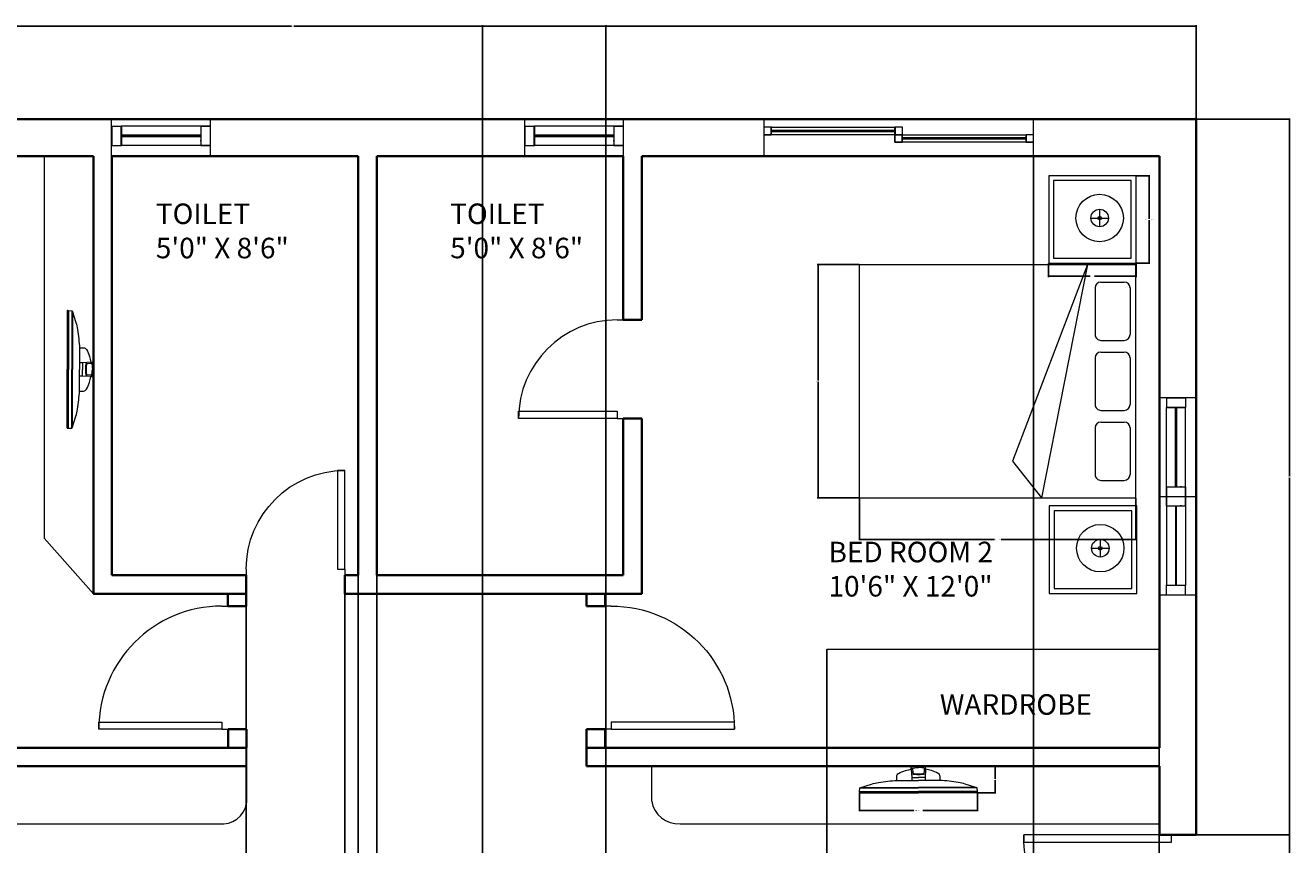
# Model space of a CAD drawing. Units: inches. Extents: x 1723 to 2209, y 1326 to 1810.
# Tile 6 of 6: x 1901 to 2209, y 1610 to 1810. Entities that reach past the tile are written whole.
import ezdxf

# ---------------------------------------------------------------- set-up
doc = ezdxf.new("R2010")
doc.units = ezdxf.units.IN
doc.layers.get('Defpoints').update_dxf_attribs({"color": 255})
for name, color, linetype, lineweight in [('A-ANNO-DIMS', 2, 'Continuous', 18), ('A-ANNO-TEXT', 7, 'Continuous', 18), ('A-AREA-IDEN', 7, 'Continuous', 18), ('A-DOOR', 3, 'Continuous', 18), ('A-EQPM', 8, 'Continuous', 13), ('A-FLOR-CASE', 9, 'Continuous', 18), ('A-FURN', 8, 'Continuous', 13), ('A-GLAZ', 4, 'Continuous', 18), ('A-WALL', 7, 'Continuous', 35), ('Sliding Door', 3, 'Continuous', 18)]:
    doc.layers.add(name, color=color, linetype=linetype, lineweight=lineweight)
doc.styles.get("Standard").update_dxf_attribs({"font": 'arial.ttf'})
doc.dimstyles.get("Standard").update_dxf_attribs({"dimtxt": 0.18, "dimasz": 0.18, "dimexe": 0.18, "dimexo": 0.0625, "dimgap": 0.09, "dimtad": 0, "dimtih": 1, "dimtoh": 1, "dimdec": 4, "dimzin": 0, "dimdsep": 46, "dimtxsty": 'Standard', "dimcen": 0.09, "dimadec": 0, "dimazin": 0, "dimtfac": 1, "dimtdec": 4, "dimtofl": 0, "dimtmove": 0, "dimatfit": 3, "dimfxl": 1, "dimtolj": 1, "dimtzin": 0, "dimarcsym": 0})

# ---------------------------------------------------------------- blocks, each defined once
blk = doc.blocks.new('B1')
at = {"color": 0}
for points in [[(-24.5, 37.9), (-24.5, 43.2, -0.236854), (-23.9, 44.5, -0.069077), (0, 47.8, -0.069077)], [(-24.5, 37.7), (-24.5, 38.9, -0.236854), (-23.9, 40.2, -0.069077), (0, 43.6, -0.069077)], [(24.5, 37.9), (24.5, 43.2, 0.236854), (23.9, 44.5, 0.069077), (0, 47.8, 0.069077)], [(24.5, 37.7), (24.5, 38.9, 0.236854), (23.9, 40.2, 0.069077), (0, 43.6, 0.069077)], [(-200, -38.4), (-200, -37.7), (-199.2, -25.8, -0.303983), (-198.5, -24.8), (-159.1, -12.4, -0.039649), (-135.4, -7, -0.017831), (-72.5, 0), (0, 0)], [(-73.6, -0.1), (-73.6, 13.1, -0.272026), (-67.3, 23.9, -0.059641), (-43.9, 33.5, -0.024069), (-24.5, 37.9), (-22.7, 10), (-22.7, 0)], [(200, -38.4), (200, -37.7), (199.2, -25.8, 0.303983), (198.5, -24.8), (159.1, -12.4, 0.039649), (135.4, -7, 0.017831), (72.5, 0), (0, 0)], [(73.6, -0.1), (73.6, 13.1, 0.272026), (67.3, 23.9, 0.059641), (43.9, 33.5, 0.024069), (24.5, 37.9), (22.7, 10), (22.7, 0)]]:
    blk.add_lwpolyline(points, format="xyb", dxfattribs=at)
for points in [[(-22.7, 10), (0, 10)], [(-19.8, 40.1), (-18.9, 26.4)], [(22.7, 10), (0, 10)], [(19.8, 40.1), (18.9, 26.4)], [(-200, -37.8), (0, -37.8)], [(-200, -41.4), (-200, -38.4), (200, -38.4)], [(-200, -38.4), (0, -38.4)], [(200, -41.4), (200, -38.4), (-200, -38.4)], [(-199.2, -25.8), (0, -25.8)], [(-198.9, -42.4), (0, -42.4)], [(-196.3, -24.2), (0, -24.2)], [(196.3, -24.2), (0, -24.2)], [(199.2, -25.8), (0, -25.8)], [(200, -37.8), (0, -37.8)], [(200, -38.4), (0, -38.4)], [(198.9, -42.4), (0, -42.4)]]:
    blk.add_lwpolyline(points, dxfattribs=at)
for centre, radius, start, end in [((0, 150), 130, 259.5789, 270), ((-15.4, 26.6), 3.53, 183.678, 262.9963), ((0, 152.2), 130, 262.9963, 270), ((0, 152.2), 130, 270, 277.0037), ((0, 150), 130, 270, 280.4211), ((15.4, 26.6), 3.53, 277.0037, 356.322), ((-198.9, -41.4), 1.06, 180, 270), ((198.9, -41.4), 1.06, 270, 0)]:
    blk.add_arc(centre, radius, start, end, dxfattribs=at)
blk = doc.blocks.new('A$C793B20D3')
for p, q in [((0.625, -0.395), (0.625, 1.975)), ((2.625, 1.975), (0.625, 1.975)), ((2.625, -0.395), (2.625, 1.975)), ((0.775, 1.675), (0.775, 1.875)), ((0.825, 1.925), (1.225, 1.925)), ((1.275, 1.675), (1.275, 1.875)), ((1.375, 1.675), (1.375, 1.875)), ((1.425, 1.925), (1.825, 1.925)), ((1.875, 1.675), (1.875, 1.875)), ((1.975, 1.675), (1.975, 1.875)), ((2.025, 1.925), (2.425, 1.925)), ((2.475, 1.675), (2.475, 1.875)), ((0.626, 1.56), (2.311, 0.917)), ((0.626, 1.56), (2.625, 1.165)), ((0.825, 1.625), (1.225, 1.625)), ((1.425, 1.625), (1.825, 1.625)), ((2.025, 1.625), (2.425, 1.625)), ((2.311, 0.917), (2.625, 1.165)), ((2.625, -0.395), (0.625, -0.395))]:
    blk.add_line(p, q)
for centre, start, end in [((0.825, 1.875), 90, 180), ((1.225, 1.875), 0, 90), ((1.425, 1.875), 90, 180), ((1.825, 1.875), 0, 90), ((2.025, 1.875), 90, 180), ((2.425, 1.875), 0, 90), ((0.825, 1.675), 180, 270), ((1.225, 1.675), 270, 0), ((1.425, 1.675), 180, 270), ((1.825, 1.675), 270, 0), ((2.025, 1.675), 180, 270), ((2.425, 1.675), 270, 0)]:
    blk.add_arc(centre, 0.05, start, end)
blk = doc.blocks.new('*U40')
for p, q in [((0, 0), (0, -6)), ((30, 0), (30, -6))]:
    blk.add_line(p, q)
blk.add_lwpolyline([(0, 0), (0, 30), (1.75, 30), (1.75, 0)], close=True)
blk.add_arc((0, 0), 30, 0, 90)
blk = doc.blocks.new('*U39')
for p, q in [((0, 0), (0, -6)), ((24, 0), (24, -6))]:
    blk.add_line(p, q)
blk.add_lwpolyline([(0, 0), (0, 24), (1.75, 24), (1.75, 0)], close=True)
blk.add_arc((0, 0), 24, 0, 90)
blk = doc.blocks.new('*U41')
for p, q in [((0, 0), (0, -6)), ((36, 0), (36, -6))]:
    blk.add_line(p, q)
blk.add_lwpolyline([(0, 0), (0, 36), (1.75, 36), (1.75, 0)], close=True)
blk.add_arc((0, 0), 36, 0, 90)
blk = doc.blocks.new('A$C7a76cbd6')
at = {"layer": 'Sliding Door'}
for p, q in [((540, 284, 0), (478, 284, 0)), ((478, 284, 0), (540, 284, 0)), ((478, 222, 0), (540, 222, 0)), ((478, 222, 0), (540, 222, 0)), ((540, 222, 0), (540, 284, 0)), ((540, 284, 0), (1585, 284, 0)), ((540, 284, 0), (540, 222, 0)), ((1585, 257, 0), (540, 257, 0)), ((540, 257, 0), (540, 249, 0)), ((540, 253, 0), (1584, 253, 0)), ((540, 249, 0), (1585, 249, 0)), ((1584, 222, 0), (540, 222, 0)), ((1584, 284, 0), (1647, 284, 0)), ((1584, 284, 0), (1584, 222, 0)), ((1646, 222, 0), (1584, 222, 0)), ((1584, 222, 0), (1584, 159, 0)), ((1584, 222, 0), (1647, 222, 0)), ((1584, 222, 0), (1647, 222, 0)), ((1584, 222, 0), (1584, 159, 0)), ((1647, 284, 0), (1585, 284, 0)), ((1585, 284, 0), (1585, 222, 0)), ((1585, 249, 0), (1585, 257, 0)), ((1585, 222, 0), (1647, 222, 0)), ((1646, 159, 0), (1646, 222, 0)), ((1647, 222, 0), (1647, 284, 0)), ((1647, 284, 0), (1647, 222, 0)), ((1647, 222, 0), (2691, 222, 0)), ((1647, 222, 0), (1647, 159, 0)), ((2690, 222, 0), (2753, 222, 0)), ((2690, 222, 0), (2690, 159, 0)), ((2753, 222, 0), (2691, 222, 0)), ((2691, 222, 0), (2691, 159, 0)), ((1584, 159, 0), (1646, 159, 0)), ((1584, 159, 0), (1647, 159, 0)), ((2691, 159, 0), (1646, 159, 0)), ((2691, 194, 0), (1647, 194, 0)), ((1647, 194, 0), (1647, 187, 0)), ((1647, 190, 0), (2690, 190, 0)), ((1647, 187, 0), (2691, 187, 0)), ((2690, 159, 0), (2753, 159, 0)), ((2691, 187, 0), (2691, 194, 0)), ((2691, 159, 0), (2753, 159, 0))]:
    blk.add_line(p, q, dxfattribs=at)
blk = doc.blocks.new('SW')
blk.add_line((2331.37, 1559.31), (2331.37, 1550.31))
at = {"layer": 'Sliding Door'}
for p, q in [((2285.07, 1559.31), (2285.07, 1550.31)), ((2285.07, 1559.31), (2285.07, 1550.31)), ((2285.07, 1559.31), (2289.58, 1559.31)), ((2289.51, 1550.31), (2289.51, 1559.31)), ((2331.37, 1559.31), (2289.51, 1559.31)), ((2289.58, 1559.31), (2289.58, 1550.31)), ((2326.86, 1555.09), (2289.58, 1555.09)), ((2289.58, 1554.81), (2326.86, 1554.81)), ((2289.58, 1554.53), (2326.86, 1554.53)), ((2326.86, 1559.31), (2326.86, 1550.31)), ((2326.86, 1559.31), (2331.37, 1559.31)), ((2326.93, 1559.31), (2326.93, 1550.31)), ((2285.07, 1550.31), (2289.51, 1550.31)), ((2285.07, 1550.31), (2289.58, 1550.31)), ((2331.37, 1550.31), (2289.51, 1550.31)), ((2289.58, 1552.81), (2289.58, 1552.25)), ((2326.86, 1550.31), (2331.37, 1550.31)), ((2326.93, 1552.25), (2326.93, 1552.81)), ((2326.93, 1550.31), (2331.37, 1550.31))]:
    blk.add_line(p, q, dxfattribs=at)
blk = doc.blocks.new('TABLE-END-LARGE')
for p, q in [((12.41, 13.14), (12.41, 8.85)), ((10.27, 10.99), (14.56, 10.99))]:
    blk.add_line(p, q)
for points in [[(21.29, 21.29), (0, 21.29), (0, 0), (21.29, 0)], [(20.1, 20.1), (1.18, 20.1), (1.18, 1.18), (20.1, 1.18)]]:
    blk.add_lwpolyline(points, close=True)
for radius in [5.77, 2.14, 0.445]:
    blk.add_circle((12.41, 10.99), radius)
blk = doc.blocks.new('*D61')
at = {"layer": 'A-ANNO-DIMS', "color": 0, "lineweight": -2, "transparency": 16777216}
for p, q in [((2103.62, 1622.66), (2103.62, 1618.24)), ((2132.3, 1622.66), (2132.3, 1618.24)), ((2103.8, 1618.42), (2116.87, 1618.42)), ((2132.12, 1618.42), (2119.05, 1618.42))]:
    blk.add_line(p, q, dxfattribs=at)
at = {"layer": 'A-ANNO-DIMS', "color": 0, "transparency": 16777216}
for points in [[(2103.8, 1618.45), (2103.8, 1618.39), (2103.62, 1618.42)], [(2132.12, 1618.45), (2132.12, 1618.39), (2132.3, 1618.42)]]:
    blk.add_solid(points, dxfattribs=at)
at = {"layer": 'Defpoints', "color": 0, "transparency": 16777216}
for p in [(2103.62, 1622.72), (2132.3, 1622.72), (2132.3, 1618.42)]:
    blk.add_point(p, dxfattribs=at)
at = {"layer": 'A-ANNO-DIMS', "color": 0, "transparency": 16777216, "insert": (2117.96, 1618.42), "char_height": 0.18, "attachment_point": 5}
blk.add_mtext('\\A1;SCREEN 29 TYP.', dxfattribs=at)
blk = doc.blocks.new('*D62')
at = {"layer": 'A-ANNO-DIMS', "color": 0, "lineweight": -2, "transparency": 16777216}
for p, q in [((2132.36, 1629.19), (2136.78, 1629.19)), ((2136.6, 1629.01), (2136.6, 1626.14)), ((2136.6, 1622.9), (2136.6, 1625.78)), ((2132.36, 1622.72), (2136.78, 1622.72))]:
    blk.add_line(p, q, dxfattribs=at)
at = {"layer": 'A-ANNO-DIMS', "color": 0, "transparency": 16777216}
for points in [[(2136.57, 1629.01), (2136.63, 1629.01), (2136.6, 1629.19)], [(2136.57, 1622.9), (2136.63, 1622.9), (2136.6, 1622.72)]]:
    blk.add_solid(points, dxfattribs=at)
at = {"layer": 'Defpoints', "color": 0, "transparency": 16777216}
for p in [(2132.3, 1629.19), (2136.6, 1629.19), (2132.3, 1622.72)]:
    blk.add_point(p, dxfattribs=at)
at = {"layer": 'A-ANNO-DIMS', "color": 0, "transparency": 16777216, "insert": (2136.6, 1625.96), "char_height": 0.18, "attachment_point": 5}
blk.add_mtext('\\A1;6 TYP.', dxfattribs=at)
blk = doc.blocks.new('*D67')
at = {"layer": 'A-ANNO-DIMS', "color": 0, "lineweight": -2, "transparency": 16777216}
for p, q in [((2171.01, 1772.94), (2174.32, 1772.94)), ((2174.14, 1772.76), (2174.14, 1762.47)), ((2174.14, 1751.83), (2174.14, 1762.11)), ((2171.01, 1751.65), (2174.32, 1751.65))]:
    blk.add_line(p, q, dxfattribs=at)
at = {"layer": 'A-ANNO-DIMS', "color": 0, "transparency": 16777216}
for points in [[(2174.11, 1772.76), (2174.17, 1772.76), (2174.14, 1772.94)], [(2174.11, 1751.83), (2174.17, 1751.83), (2174.14, 1751.65)]]:
    blk.add_solid(points, dxfattribs=at)
at = {"layer": 'Defpoints', "color": 0, "transparency": 16777216}
for p in [(2170.95, 1772.94), (2174.14, 1772.94), (2170.95, 1751.65)]:
    blk.add_point(p, dxfattribs=at)
at = {"layer": 'A-ANNO-DIMS', "color": 0, "transparency": 16777216, "insert": (2174.14, 1762.29), "char_height": 0.18, "attachment_point": 5}
blk.add_mtext('\\A1;END TABLE 21 TYP.', dxfattribs=at)
blk = doc.blocks.new('*D68')
at = {"layer": 'A-ANNO-DIMS', "color": 0, "lineweight": -2, "transparency": 16777216}
for p, q in [((2149.66, 1751.59), (2149.66, 1748.28)), ((2170.95, 1751.59), (2170.95, 1748.28)), ((2149.84, 1748.46), (2159.78, 1748.46)), ((2170.77, 1748.46), (2160.84, 1748.46))]:
    blk.add_line(p, q, dxfattribs=at)
at = {"layer": 'A-ANNO-DIMS', "color": 0, "transparency": 16777216}
for points in [[(2149.84, 1748.49), (2149.84, 1748.43), (2149.66, 1748.46)], [(2170.77, 1748.49), (2170.77, 1748.43), (2170.95, 1748.46)]]:
    blk.add_solid(points, dxfattribs=at)
at = {"layer": 'Defpoints', "color": 0, "transparency": 16777216}
for p in [(2149.66, 1751.65), (2170.95, 1751.65), (2170.95, 1748.46)]:
    blk.add_point(p, dxfattribs=at)
at = {"layer": 'A-ANNO-DIMS', "color": 0, "transparency": 16777216, "insert": (2160.31, 1748.46), "char_height": 0.18, "attachment_point": 5}
blk.add_mtext('\\A1;21 TYP.', dxfattribs=at)
blk = doc.blocks.new('*D71')
at = {"layer": 'A-ANNO-DIMS', "color": 0, "lineweight": -2, "transparency": 16777216}
for p, q in [((2103.61, 1694.46), (2103.61, 1684.25)), ((2170.9, 1694.46), (2170.9, 1684.25)), ((2103.79, 1684.43), (2136.44, 1684.43)), ((2170.72, 1684.43), (2138.07, 1684.43))]:
    blk.add_line(p, q, dxfattribs=at)
at = {"layer": 'A-ANNO-DIMS', "color": 0, "transparency": 16777216}
for points in [[(2103.79, 1684.46), (2103.79, 1684.4), (2103.61, 1684.43)], [(2170.72, 1684.46), (2170.72, 1684.4), (2170.9, 1684.43)]]:
    blk.add_solid(points, dxfattribs=at)
at = {"layer": 'Defpoints', "color": 0, "transparency": 16777216}
for p in [(2103.61, 1694.52), (2170.9, 1694.52), (2170.9, 1684.43)]:
    blk.add_point(p, dxfattribs=at)
at = {"layer": 'A-ANNO-DIMS', "color": 0, "transparency": 16777216, "insert": (2137.26, 1684.43), "char_height": 0.18, "attachment_point": 5}
blk.add_mtext('\\A1;BED 67 TYP.', dxfattribs=at)
blk = doc.blocks.new('*D72')
at = {"layer": 'A-ANNO-DIMS', "color": 0, "lineweight": -2, "transparency": 16777216}
for p, q in [((2103.55, 1751.32), (2093.34, 1751.32)), ((2093.52, 1751.14), (2093.52, 1723.1)), ((2093.52, 1694.7), (2093.52, 1722.74)), ((2103.55, 1694.52), (2093.34, 1694.52))]:
    blk.add_line(p, q, dxfattribs=at)
at = {"layer": 'A-ANNO-DIMS', "color": 0, "transparency": 16777216}
for points in [[(2093.49, 1751.14), (2093.55, 1751.14), (2093.52, 1751.32)], [(2093.49, 1694.7), (2093.55, 1694.7), (2093.52, 1694.52)]]:
    blk.add_solid(points, dxfattribs=at)
at = {"layer": 'Defpoints', "color": 0, "transparency": 16777216}
for p in [(2103.61, 1751.32), (2093.52, 1694.52), (2103.61, 1694.52)]:
    blk.add_point(p, dxfattribs=at)
at = {"layer": 'A-ANNO-DIMS', "color": 0, "transparency": 16777216, "insert": (2093.52, 1722.92), "char_height": 0.18, "attachment_point": 5}
blk.add_mtext('\\A1;57 TYP.', dxfattribs=at)
blk = doc.blocks.new('*D93')
at = {"layer": 'A-ANNO-DIMS', "color": 0, "lineweight": -2, "transparency": 16777216}
for p, q in [((1745.6, 1633.75), (1745.6, 1809.54)), ((1745.78, 1809.36), (1965.31, 1809.36)), ((2185.42, 1809.36), (1965.9, 1809.36)), ((2185.6, 1786.75), (2185.6, 1809.54))]:
    blk.add_line(p, q, dxfattribs=at)
at = {"layer": 'A-ANNO-DIMS', "color": 0, "transparency": 16777216}
for points in [[(1745.78, 1809.39), (1745.78, 1809.33), (1745.6, 1809.36)], [(2185.42, 1809.39), (2185.42, 1809.33), (2185.6, 1809.36)]]:
    blk.add_solid(points, dxfattribs=at)
at = {"layer": 'Defpoints', "color": 0, "transparency": 16777216}
for p in [(2185.6, 1809.36), (2185.6, 1786.69), (1745.6, 1633.69)]:
    blk.add_point(p, dxfattribs=at)
at = {"layer": 'A-ANNO-DIMS', "color": 0, "transparency": 16777216, "insert": (1965.6, 1809.36), "char_height": 0.18, "attachment_point": 5}
blk.add_mtext('\\A1;440', dxfattribs=at)
blk = doc.blocks.new('*D101')
at = {"layer": 'A-ANNO-DIMS', "color": 0, "lineweight": -2, "transparency": 16777216}
for p, q in [((2185.67, 1786.69), (2208.45, 1786.69)), ((2208.27, 1786.51), (2208.27, 1699.77)), ((2208.27, 1612.67), (2208.27, 1699.41)), ((2185.67, 1612.49), (2208.45, 1612.49))]:
    blk.add_line(p, q, dxfattribs=at)
at = {"layer": 'A-ANNO-DIMS', "color": 0, "transparency": 16777216}
for points in [[(2208.24, 1786.51), (2208.3, 1786.51), (2208.27, 1786.69)], [(2208.24, 1612.67), (2208.3, 1612.67), (2208.27, 1612.49)]]:
    blk.add_solid(points, dxfattribs=at)
at = {"layer": 'Defpoints', "color": 0, "transparency": 16777216}
for p in [(2185.6, 1786.69), (2208.27, 1786.69), (2185.6, 1612.49)]:
    blk.add_point(p, dxfattribs=at)
at = {"layer": 'A-ANNO-DIMS', "color": 0, "transparency": 16777216, "insert": (2208.27, 1699.59), "char_height": 0.18, "attachment_point": 5}
blk.add_mtext('\\A1;174.2', dxfattribs=at)
blk = doc.blocks.new('*D102')
at = {"layer": 'A-ANNO-DIMS', "color": 0, "lineweight": -2, "transparency": 16777216}
for p, q in [((2185.67, 1612.49), (2208.45, 1612.49)), ((2208.27, 1612.31), (2208.27, 1594.67)), ((2208.27, 1576.67), (2208.27, 1594.3)), ((2185.67, 1576.49), (2208.45, 1576.49))]:
    blk.add_line(p, q, dxfattribs=at)
at = {"layer": 'A-ANNO-DIMS', "color": 0, "transparency": 16777216}
for points in [[(2208.24, 1612.31), (2208.3, 1612.31), (2208.27, 1612.49)], [(2208.24, 1576.67), (2208.3, 1576.67), (2208.27, 1576.49)]]:
    blk.add_solid(points, dxfattribs=at)
at = {"layer": 'Defpoints', "color": 0, "transparency": 16777216}
for p in [(2185.6, 1612.49), (2208.27, 1612.49), (2185.6, 1576.49)]:
    blk.add_point(p, dxfattribs=at)
at = {"layer": 'A-ANNO-DIMS', "color": 0, "transparency": 16777216, "insert": (2208.27, 1594.49), "char_height": 0.18, "attachment_point": 5}
blk.add_mtext('\\A1;36', dxfattribs=at)
blk = doc.blocks.new('*D107')
at = {"layer": 'A-ANNO-DIMS', "color": 0, "lineweight": -2, "transparency": 16777216}
for p, q in [((2011.84, 1506.25), (2011.84, 1809.54)), ((2012.02, 1809.36), (2026.63, 1809.36)), ((2041.66, 1809.36), (2027.06, 1809.36)), ((2041.84, 1506.25), (2041.84, 1809.54))]:
    blk.add_line(p, q, dxfattribs=at)
at = {"layer": 'A-ANNO-DIMS', "color": 0, "transparency": 16777216}
for points in [[(2012.02, 1809.39), (2012.02, 1809.33), (2011.84, 1809.36)], [(2041.66, 1809.39), (2041.66, 1809.33), (2041.84, 1809.36)]]:
    blk.add_solid(points, dxfattribs=at)
at = {"layer": 'Defpoints', "color": 0, "transparency": 16777216}
for p in [(2041.84, 1809.36), (2011.84, 1506.19), (2041.84, 1506.19)]:
    blk.add_point(p, dxfattribs=at)
at = {"layer": 'A-ANNO-DIMS', "color": 0, "transparency": 16777216, "insert": (2026.84, 1809.36), "char_height": 0.18, "attachment_point": 5}
blk.add_mtext('\\A1;30', dxfattribs=at)
blk = doc.blocks.new('*D108')
at = {"layer": 'A-ANNO-DIMS', "color": 0, "lineweight": -2, "transparency": 16777216}
for p, q in [((1954.3, 1671.13), (1954.3, 1325.84)), ((1978.3, 1671.13), (1978.3, 1325.84)), ((1954.48, 1326.02), (1966.08, 1326.02)), ((1978.12, 1326.02), (1966.52, 1326.02))]:
    blk.add_line(p, q, dxfattribs=at)
at = {"layer": 'A-ANNO-DIMS', "color": 0, "transparency": 16777216}
for points in [[(1954.48, 1326.05), (1954.48, 1325.99), (1954.3, 1326.02)], [(1978.12, 1326.05), (1978.12, 1325.99), (1978.3, 1326.02)]]:
    blk.add_solid(points, dxfattribs=at)
at = {"layer": 'Defpoints', "color": 0, "transparency": 16777216}
for p in [(1954.3, 1671.19), (1978.3, 1671.19), (1978.3, 1326.02)]:
    blk.add_point(p, dxfattribs=at)
at = {"layer": 'A-ANNO-DIMS', "color": 0, "transparency": 16777216, "insert": (1966.3, 1326.02), "char_height": 0.18, "attachment_point": 5}
blk.add_mtext('\\A1;24', dxfattribs=at)
blk = doc.blocks.new('*D109')
at = {"layer": 'A-ANNO-DIMS', "color": 0, "lineweight": -2, "transparency": 16777216}
for p, q in [((1981.6, 1777.63), (1981.6, 1325.84)), ((1986.1, 1777.63), (1986.1, 1325.84)), ((1981.78, 1326.02), (1983.6, 1326.02)), ((1985.92, 1326.02), (1984.11, 1326.02))]:
    blk.add_line(p, q, dxfattribs=at)
at = {"layer": 'A-ANNO-DIMS', "color": 0, "transparency": 16777216}
for points in [[(1981.78, 1326.05), (1981.78, 1325.99), (1981.6, 1326.02)], [(1985.92, 1326.05), (1985.92, 1325.99), (1986.1, 1326.02)]]:
    blk.add_solid(points, dxfattribs=at)
at = {"layer": 'Defpoints', "color": 0, "transparency": 16777216}
for p in [(1981.6, 1777.69), (1986.1, 1777.69), (1986.1, 1326.02)]:
    blk.add_point(p, dxfattribs=at)
at = {"layer": 'A-ANNO-DIMS', "color": 0, "transparency": 16777216, "insert": (1983.85, 1326.02), "char_height": 0.18, "attachment_point": 5}
blk.add_mtext('\\A1;4.5', dxfattribs=at)
blk = doc.blocks.new('*D113')
at = {"layer": 'A-ANNO-DIMS', "color": 0, "lineweight": -2, "transparency": 16777216}
for p, q in [((2095.65, 1657.63), (2095.65, 1325.84)), ((2176.6, 1657.63), (2176.6, 1325.84)), ((2095.83, 1326.02), (2135.73, 1326.02)), ((2176.42, 1326.02), (2136.52, 1326.02))]:
    blk.add_line(p, q, dxfattribs=at)
at = {"layer": 'A-ANNO-DIMS', "color": 0, "transparency": 16777216}
for points in [[(2095.83, 1326.05), (2095.83, 1325.99), (2095.65, 1326.02)], [(2176.42, 1326.05), (2176.42, 1325.99), (2176.6, 1326.02)]]:
    blk.add_solid(points, dxfattribs=at)
at = {"layer": 'Defpoints', "color": 0, "transparency": 16777216}
for p in [(2095.65, 1657.69), (2176.6, 1657.69), (2176.6, 1326.02)]:
    blk.add_point(p, dxfattribs=at)
at = {"layer": 'A-ANNO-DIMS', "color": 0, "transparency": 16777216, "insert": (2136.13, 1326.02), "char_height": 0.18, "attachment_point": 5}
blk.add_mtext('\\A1;80.95', dxfattribs=at)
blk = doc.blocks.new('*D115')
at = {"layer": 'A-ANNO-DIMS', "color": 0, "lineweight": -2, "transparency": 16777216}
for p, q in [((2145.93, 1777.63), (2145.93, 1325.84)), ((2176.6, 1777.63), (2176.6, 1325.84)), ((2146.11, 1326.02), (2160.8, 1326.02)), ((2176.42, 1326.02), (2161.73, 1326.02))]:
    blk.add_line(p, q, dxfattribs=at)
at = {"layer": 'A-ANNO-DIMS', "color": 0, "transparency": 16777216}
for points in [[(2146.11, 1326.05), (2146.11, 1325.99), (2145.93, 1326.02)], [(2176.42, 1326.05), (2176.42, 1325.99), (2176.6, 1326.02)]]:
    blk.add_solid(points, dxfattribs=at)
at = {"layer": 'Defpoints', "color": 0, "transparency": 16777216}
for p in [(2145.93, 1777.69), (2176.6, 1777.69), (2176.6, 1326.02)]:
    blk.add_point(p, dxfattribs=at)
at = {"layer": 'A-ANNO-DIMS', "color": 0, "transparency": 16777216, "insert": (2161.26, 1326.02), "char_height": 0.18, "attachment_point": 5}
blk.add_mtext('\\A1;30.677', dxfattribs=at)

msp = doc.modelspace()

# ---------------------------------------------------------------- linework, layer by layer
at = {"layer": 'A-FLOR-CASE'}
for p, q in [((1905.1032, 1777.6915), (1905.1032, 1684.7482)), ((1917.1032, 1671.1915), (1905.1032, 1684.7482)), ((2095.6512, 1657.6915), (2176.6032, 1657.6915)), ((2095.6512, 1657.6915), (2095.6512, 1633.6915)), ((1954.4027, 1633.6915), (1954.4027, 1620.2942)), ((2053.0254, 1620.7052), (2053.0254, 1629.1915)), ((1816.6032, 1615.1915), (1947.6384, 1615.1915)), ((2059.9278, 1615.1915), (2176.6032, 1615.1915))]:
    msp.add_line(p, q, dxfattribs=at)
for centre, radius, start, end in [((2059.5064, 1621.7412), 6.5632, 189.081939, 273.681267), ((1948.4253, 1621.1832), 6.0431, 262.51773, 351.540582)]:
    msp.add_arc(centre, radius, start, end, dxfattribs=at)
at = {"layer": 'A-GLAZ'}
for p, q in [((2080.3457, 1786.6915), (2080.3457, 1777.6915)), ((2145.9265, 1786.6915), (2145.9265, 1777.6915))]:
    msp.add_line(p, q, dxfattribs=at)
for points in [[(1921.558, 1786.6915), (1945.558, 1786.6915), (1945.558, 1777.6915), (1921.558, 1777.6915)], [(2022.1032, 1786.6915), (2046.1032, 1786.6915), (2046.1032, 1777.6915), (2022.1032, 1777.6915)], [(2176.6032, 1718.8784), (2176.6032, 1694.8784), (2185.6032, 1694.8784), (2185.6032, 1718.8784)], [(2176.6032, 1670.8784), (2176.6032, 1694.8784), (2185.6032, 1694.8784), (2185.6032, 1670.8784)]]:
    msp.add_lwpolyline(points, close=True, dxfattribs=at)
at = {"layer": 'A-WALL'}
for p, q in [((1797.1032, 1777.6915), (1917.1032, 1777.6915)), ((1917.1032, 1777.6915), (1917.1032, 1671.1915)), ((1921.6032, 1777.6915), (1921.6032, 1675.6915)), ((1921.6032, 1777.6915), (1981.6032, 1777.6915)), ((1981.6032, 1777.6915), (1981.6032, 1675.6915)), ((1986.1032, 1777.6915), (1986.1032, 1675.6915)), ((1986.1032, 1777.6915), (2046.1032, 1777.6915)), ((2046.1032, 1777.6915), (2046.1032, 1737.8413)), ((2050.6032, 1777.6915), (2050.6032, 1737.8413)), ((2050.6032, 1777.6915), (2176.6032, 1777.6915)), ((2176.6032, 1777.6915), (2176.6032, 1633.6915)), ((2046.1032, 1737.8413), (2050.6032, 1737.8413)), ((2046.1032, 1713.8413), (2050.6032, 1713.8413)), ((2046.1032, 1713.8413), (2046.1032, 1675.6915)), ((2050.6032, 1713.8413), (2050.6032, 1671.1915)), ((1921.6032, 1675.6915), (1954.3022, 1675.6915)), ((1954.3022, 1675.6915), (1954.3022, 1671.1915)), ((1978.3022, 1675.6915), (1978.3022, 1671.1915)), ((1978.3022, 1675.6915), (1981.6032, 1675.6915)), ((1986.1032, 1675.6915), (2046.1032, 1675.6915)), ((1917.1032, 1671.1915), (1954.3022, 1671.1915)), ((1949.8022, 1668.1915), (1949.8022, 1671.1915)), ((1954.3022, 1668.1915), (1954.3022, 1671.1915)), ((1978.3022, 1671.1915), (2050.6032, 1671.1915)), ((2037.1788, 1668.1915), (2037.1788, 1671.1915)), ((2041.6788, 1668.1915), (2041.6788, 1671.1915)), ((1949.8022, 1668.1915), (1954.3022, 1668.1915)), ((2037.1788, 1668.1915), (2041.6788, 1668.1915)), ((1949.9027, 1638.1915), (1949.9027, 1633.6915)), ((1954.4027, 1638.1915), (1949.9027, 1638.1915)), ((1954.4027, 1638.1915), (1954.4027, 1633.6915)), ((2037.1788, 1638.1915), (2037.1788, 1633.6915)), ((2041.6788, 1638.1915), (2037.1788, 1638.1915)), ((2041.6788, 1638.1915), (2041.6788, 1633.6915)), ((1797.1032, 1633.6915), (1954.4027, 1633.6915)), ((2037.1788, 1633.6915), (2037.1788, 1629.1915)), ((2037.1788, 1633.6915), (2176.6032, 1633.6915)), ((1816.6032, 1629.1915), (1954.4027, 1629.1915)), ((2037.1788, 1629.1915), (2176.6032, 1629.1915)), ((2176.6032, 1629.1915), (2176.6032, 1612.485)), ((2176.6032, 1612.485), (2185.6032, 1612.485))]:
    msp.add_line(p, q, dxfattribs=at)
msp.add_lwpolyline([(1788.1032, 1629.1915), (1788.1032, 1786.6915), (2185.6032, 1786.6915), (2185.6032, 1612.485)], dxfattribs=at)

# ---------------------------------------------------------------- block references
at = {"layer": 'A-DOOR', "rotation": 90}
for name, p in [('*U39', (2044.6032, 1713.8413)), ('*U40', (1948.4027, 1638.1915))]:
    msp.add_blockref(name, p, dxfattribs=at)
at = {"layer": 'A-DOOR', "xscale": -1}
msp.add_blockref('*U39', (1978.3022, 1677.1915), dxfattribs=at)
for name, p, rotation in [('*U40', (2043.1788, 1638.1915), 270), ('*U41', (2179.6032, 1612.485), 89.99999999999936)]:
    msp.add_blockref(name, p, dxfattribs=dict(at, rotation=rotation))
at = {"layer": 'A-EQPM', "xscale": 0.0716950546847252, "yscale": 0.0716950546847252, "zscale": 0.0716950546847252, "rotation": 270}
msp.add_blockref('B1', (1913.7358, 1725.804), dxfattribs=at)
at = {"layer": 'A-EQPM', "xscale": 0.0716950546847252, "yscale": 0.0716950546847252, "zscale": 0.0716950546847252}
msp.add_blockref('B1', (2117.9599, 1625.7645), dxfattribs=at)
at = {"layer": 'A-FURN'}
for p in [(2149.6634, 1751.6501), (2149.8173, 1671.2802)]:
    msp.add_blockref('TABLE-END-LARGE', p, dxfattribs=at)
at = {"layer": 'A-FURN', "xscale": 28.39623388090672, "yscale": 28.39623388090672, "zscale": 28.39623388090672, "rotation": 270}
msp.add_blockref('A$C793B20D3', (2114.8164, 1769.0632), dxfattribs=at)
at = {"layer": 'A-GLAZ', "xscale": 0.5174661543078929, "yscale": 0.5174661543078929, "zscale": 0.5174661543078929}
for p in [(739.155, 978.088), (839.7001, 978.088)]:
    msp.add_blockref('SW', p, dxfattribs=at)
at = {"layer": 'A-GLAZ'}
for name, p, xscale, yscale, zscale, rotation in [('A$C7a76cbd6', (2159.7122, 1789.309), 0.0288245099661422, 0.0288245099661422, 0.0288245099661422, 180), ('SW', (2985.2067, 2901.2814), -0.5174661543078929, 0.5174661543078929, 0.5174661543078929, 90), ('SW', (2985.2067, 488.4754), 0.5174661543078929, 0.5174661543078929, 0.5174661543078929, 90)]:
    msp.add_blockref(name, p, dxfattribs=dict(at, xscale=xscale, yscale=yscale, zscale=zscale, rotation=rotation))

# ---------------------------------------------------------------- texts
at = {"layer": 'A-ANNO-TEXT', "insert": (2123.1601, 1646.7323), "char_height": 5, "attachment_point": 1}
msp.add_mtext_dynamic_manual_height_columns('WARDROBE', width=43.999866, gutter_width=12.5, heights=[0], dxfattribs=at)
at = {"layer": 'A-AREA-IDEN', "char_height": 5, "attachment_point": 1}
for s, width, insert in [('TOILET\\P5\'0" X 8\'6"', 40.517526, (1932.308, 1766.1687)), ('TOILET\\P5\'0" X 8\'6"', 40.517526, (2003.96, 1766.1687)), ('BED ROOM 2\\P10\'6" X 12\'0"', 63.019392, (2096.059, 1683.8482))]:
    msp.add_mtext_dynamic_manual_height_columns(s, width=width, gutter_width=12.5, heights=[0], dxfattribs=dict(at, insert=insert))

# ---------------------------------------------------------------- dimensions: what is measured, and where the dimension line sits
at = {"layer": 'A-ANNO-DIMS'}
for base, p1, p2, override, picture, middle in [((2185.6032, 1809.3615), (1745.6032, 1633.6915), (2185.6032, 1786.6915), {"dimdec": 0, "dimlfac": 1, "dimrnd": 0, "dimzin": 0, "dimdsep": 46, "dimlunit": 2}, '*D93', (1965.6032, 1809.3615)), ((2041.8437, 1809.3615), (2011.8437, 1506.1915), (2041.8437, 1506.1915), {"dimdec": 0, "dimlfac": 1, "dimrnd": 0, "dimzin": 0, "dimdsep": 46, "dimlunit": 2}, '*D107', (2026.8437, 1809.3615)), ((1986.1032, 1326.0215), (1981.6032, 1777.6915), (1986.1032, 1777.6915), {"dimdec": 1, "dimlfac": 1, "dimrnd": 0, "dimzin": 0, "dimdsep": 46, "dimlunit": 2}, '*D109', (1983.8532, 1326.0215)), ((2176.6032, 1326.0215), (2145.9265, 1777.6915), (2176.6032, 1777.6915), {"dimdec": 3, "dimlfac": 1, "dimrnd": 0, "dimzin": 0, "dimdsep": 46, "dimlunit": 2}, '*D115', (2161.2649, 1326.0215)), ((1978.3022, 1326.0215), (1954.3022, 1671.1915), (1978.3022, 1671.1915), {"dimdec": 0, "dimlfac": 1, "dimrnd": 0, "dimzin": 0, "dimdsep": 46, "dimlunit": 2}, '*D108', (1966.3022, 1326.0215)), ((2176.6032, 1326.0215), (2095.6512, 1657.6915), (2176.6032, 1657.6915), {"dimdec": 2, "dimlfac": 1, "dimrnd": 0, "dimzin": 0, "dimdsep": 46, "dimlunit": 2}, '*D113', (2136.1272, 1326.0215))]:
    dim = msp.add_linear_dim(base=base, p1=p1, p2=p2, dimstyle='Standard', override=override, dxfattribs=at)
    dim.commit()
    dim.dimension.update_dxf_attribs({"geometry": picture, "text_midpoint": middle})
for base, p1, p2, override, picture, middle in [((2208.2732, 1786.6915), (2185.6032, 1612.485), (2185.6032, 1786.6915), {"dimdec": 1, "dimlfac": 1, "dimrnd": 0, "dimzin": 0, "dimdsep": 46, "dimlunit": 2}, '*D101', (2208.2732, 1699.5883)), ((2208.2732, 1612.485), (2185.6032, 1576.485), (2185.6032, 1612.485), {"dimdec": 0, "dimlfac": 1, "dimrnd": 0, "dimzin": 0, "dimdsep": 46, "dimlunit": 2}, '*D102', (2208.2732, 1594.485))]:
    dim = msp.add_linear_dim(base=base, p1=p1, p2=p2, angle=90, dimstyle='Standard', override=override, dxfattribs=at)
    dim.commit()
    dim.dimension.update_dxf_attribs({"geometry": picture, "text_midpoint": middle})
for base, p1, p2, angle, text, picture, middle in [((2174.1428, 1772.9366), (2170.9499, 1751.6501), (2170.9499, 1772.9366), 90, 'END TABLE <> TYP.', '*D67', (2174.1428, 1762.2934)), ((2093.5203, 1694.5229), (2103.6132, 1751.3154), (2103.6132, 1694.5229), 270, '<> TYP.', '*D72', (2093.5203, 1722.9192)), ((2136.6006, 1629.1915), (2132.2989, 1622.7239), (2132.2989, 1629.1915), 90, '<> TYP.', '*D62', (2136.6006, 1625.9577))]:
    dim = msp.add_linear_dim(base=base, p1=p1, p2=p2, angle=angle, text=text, dimstyle='Standard', override={"dimdec": 0, "dimlfac": 1, "dimrnd": 0, "dimzin": 0, "dimdsep": 46, "dimlunit": 2}, dxfattribs=at)
    dim.commit()
    dim.dimension.update_dxf_attribs({"geometry": picture, "text_midpoint": middle})
for base, p1, p2, text, picture, middle in [((2170.9499, 1748.4572), (2149.6634, 1751.6501), (2170.9499, 1751.6501), '<> TYP.', '*D68', (2160.3066, 1748.4572)), ((2170.8991, 1684.4301), (2103.6132, 1694.5229), (2170.8991, 1694.5229), 'BED <> TYP.', '*D71', (2137.2562, 1684.4301)), ((2132.2989, 1618.4222), (2103.6209, 1622.7239), (2132.2989, 1622.7239), 'SCREEN <> TYP.', '*D61', (2117.9599, 1618.4222))]:
    dim = msp.add_linear_dim(base=base, p1=p1, p2=p2, text=text, dimstyle='Standard', override={"dimdec": 0, "dimlfac": 1, "dimrnd": 0, "dimzin": 0, "dimdsep": 46, "dimlunit": 2}, dxfattribs=at)
    dim.commit()
    dim.dimension.update_dxf_attribs({"geometry": picture, "text_midpoint": middle})

doc.saveas('drawing.dxf')
